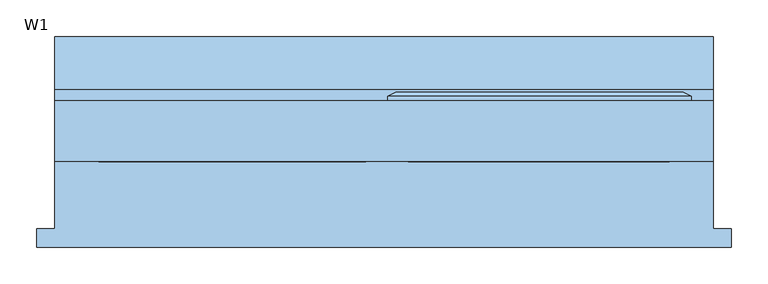
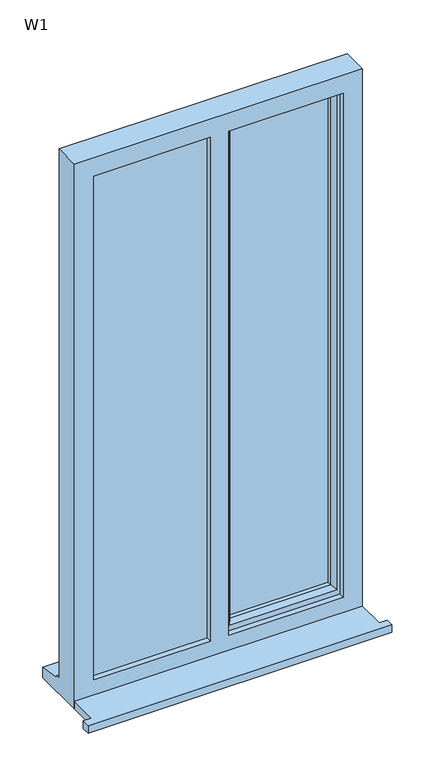
"""IFC4 building model written with IfcOpenShell, lengths in millimetres: window geometry, W1."""

from ifc_helpers import new_model, si_unit, frame, origin, place, context, project, spatial, polyline, outline, extrude, faceted_brep, source, transform, mapped, element, save


def w1_9a3d44e1(model_context):
    return source(origin(), model_context, "Body", "SolidModel", [
        extrude(outline(polyline([(-760.0, -129.0434322), (-760.0, -104.0434322), (-735.0, -104.0434322), (-735.0, -12.0434322), (165.0, -12.0434322), (165.0, -104.0434322), (190.0, -104.0434322), (190.0, -129.0434322), (-760.0, -129.0434322)])), frame((0.0, 0.0, 600.0), z_axis=(0.0, 0.0, 1.0), x_axis=(1.0, 0.0, 0.0)), (0.0, 0.0, 1.0), 25.0),
        faceted_brep([(-280.0, 70.9565678, 2370.0), (-280.0, 76.7300705, 2370.0), (-280.0, 76.7300705, 653.0), (-280.0, 70.9565678, 653.0), (-270.0, 5.9565678, 2360.0), (-270.0, 70.9565678, 2360.0), (-270.0, 70.9565678, 663.0), (-270.0, 5.9565678, 663.0), (-230.0, 20.4494677, 2320.0), (-240.1480377, 5.9565678, 2330.1480377), (-240.1480377, 5.9565678, 692.8519623), (-230.0, 20.4494677, 703.0), (-230.0, 34.9565678, 2320.0), (-230.0, 34.9565678, 703.0), (-240.0, 58.9565678, 2330.0), (-240.0, 34.9565678, 2330.0), (-240.0, 34.9565678, 693.0), (-240.0, 58.9565678, 693.0), (-230.0, 76.7300705, 2320.0), (-230.0, 58.9565678, 2320.0), (-230.0, 58.9565678, 703.0), (-230.0, 76.7300705, 703.0), (-247.4457548, 82.5035732, 2337.4457548), (-247.4457548, 82.5035732, 685.5542452), (-269.2153903, 82.5035732, 2359.2153903), (-269.2153903, 82.5035732, 663.7846097), (135.0, 76.7300705, 653.0), (135.0, 70.9565678, 653.0), (125.0, 70.9565678, 663.0), (125.0, 5.9565678, 663.0), (95.1480377, 5.9565678, 692.8519623), (85.0, 20.4494677, 703.0), (85.0, 34.9565678, 703.0), (95.0, 34.9565678, 693.0), (95.0, 58.9565678, 693.0), (85.0, 58.9565678, 703.0), (85.0, 76.7300705, 703.0), (102.4457548, 82.5035732, 685.5542452), (124.2153903, 82.5035732, 663.7846097), (135.0, 76.7300705, 2370.0), (135.0, 70.9565678, 2370.0), (125.0, 70.9565678, 2360.0), (125.0, 5.9565678, 2360.0), (95.1480377, 5.9565678, 2330.1480377), (85.0, 20.4494677, 2320.0), (85.0, 34.9565678, 2320.0), (95.0, 34.9565678, 2330.0), (95.0, 58.9565678, 2330.0), (85.0, 58.9565678, 2320.0), (85.0, 76.7300705, 2320.0), (102.4457548, 82.5035732, 2337.4457548), (124.2153903, 82.5035732, 2359.2153903)], [[[0, 1, 2, 3]], [[4, 5, 6, 7]], [[8, 9, 10, 11]], [[12, 8, 11, 13]], [[14, 15, 16, 17]], [[18, 19, 20, 21]], [[22, 18, 21, 23]], [[1, 24, 25, 2]], [[3, 2, 26, 27]], [[7, 6, 28, 29]], [[11, 10, 30, 31]], [[13, 11, 31, 32]], [[17, 16, 33, 34]], [[21, 20, 35, 36]], [[23, 21, 36, 37]], [[2, 25, 38, 26]], [[27, 26, 39, 40]], [[29, 28, 41, 42]], [[31, 30, 43, 44]], [[32, 31, 44, 45]], [[34, 33, 46, 47]], [[36, 35, 48, 49]], [[37, 36, 49, 50]], [[26, 38, 51, 39]], [[40, 39, 1, 0]], [[3, 27, 40, 0], [5, 41, 28, 6]], [[42, 41, 5, 4]], [[7, 29, 42, 4], [9, 43, 30, 10]], [[44, 43, 9, 8]], [[45, 44, 8, 12]], [[15, 46, 33, 16], [13, 32, 45, 12]], [[47, 46, 15, 14]], [[17, 34, 47, 14], [19, 48, 35, 20]], [[49, 48, 19, 18]], [[50, 49, 18, 22]], [[24, 51, 38, 25], [23, 37, 50, 22]], [[39, 51, 24, 1]]]),
        extrude(outline(polyline([(2340.0, -310.0), (2360.0, -310.0), (2360.0, -695.0), (663.0, -695.0), (663.0, -310.0), (683.0, -310.0), (683.0, -675.0), (2340.0, -675.0), (2340.0, -310.0)])), frame((0.0, 29.9565678, 0.0), z_axis=(0.0, 1.0, 0.0), x_axis=(0.0, 0.0, 1.0)), (0.0, 0.0, 1.0), 41.0),
        faceted_brep([(165.0, -12.0434322, 2400.0), (-735.0, -12.0434322, 2400.0), (-735.0, -12.0434322, 600.0), (165.0, -12.0434322, 600.0), (105.0, -12.0434322, 2340.0), (105.0, -12.0434322, 675.0), (-252.0, -12.0434322, 675.0), (-252.0, -12.0434322, 2340.0), (-310.0, -12.0434322, 2340.0), (-310.0, -12.0434322, 675.0), (-675.0, -12.0434322, 675.0), (-675.0, -12.0434322, 2340.0), (-735.0, 70.9565678, 2400.0), (-735.0, 70.9565678, 651.0), (-735.0, 85.9565678, 649.68767), (-735.0, 85.9565678, 644.7449676), (-735.0, 158.4565678, 633.8088847), (-735.0, 158.4565678, 600.0), (165.0, 70.9565678, 2400.0), (165.0, 70.9565678, 651.0), (-695.0, 70.9565678, 2360.0), (-695.0, 70.9565678, 663.0), (-310.0, 70.9565678, 663.0), (-310.0, 70.9565678, 2360.0), (-270.0, 70.9565678, 2360.0), (-270.0, 70.9565678, 663.0), (125.0, 70.9565678, 663.0), (125.0, 70.9565678, 2360.0), (-695.0, 5.9565678, 2360.0), (-695.0, 5.9565678, 663.0), (-300.0, 5.9565678, 2360.0), (-300.0, 5.9565678, 663.0), (-310.0, 5.9565678, 2340.0), (-675.0, 5.9565678, 2340.0), (-675.0, 5.9565678, 675.0), (-310.0, 5.9565678, 675.0), (-270.0, 5.9565678, 2360.0), (125.0, 5.9565678, 2360.0), (125.0, 5.9565678, 663.0), (-270.0, 5.9565678, 663.0), (105.0, 5.9565678, 2340.0), (-252.0, 5.9565678, 2340.0), (-252.0, 5.9565678, 675.0), (105.0, 5.9565678, 675.0), (-310.0, 29.9565678, 2360.0), (-300.0, 29.9565678, 2360.0), (165.0, 158.4565678, 600.0), (165.0, 158.4565678, 633.8088847), (165.0, 85.9565678, 644.7449676), (165.0, 85.9565678, 649.68767), (-300.0, 29.9565678, 663.0), (-310.0, 29.9565678, 663.0)], [[[0, 1, 2, 3], [4, 5, 6, 7], [8, 9, 10, 11]], [[2, 1, 12, 13, 14, 15, 16, 17]], [[13, 12, 18, 19], [20, 21, 22, 23], [24, 25, 26, 27]], [[21, 20, 28, 29]], [[28, 30, 31, 29], [32, 33, 34, 35]], [[36, 37, 38, 39], [40, 41, 42, 43]], [[33, 11, 10, 34]], [[1, 0, 18, 12]], [[28, 20, 23, 44, 45, 30]], [[27, 37, 36, 24]], [[11, 33, 32, 8]], [[40, 4, 7, 41]], [[19, 18, 0, 3, 46, 47, 48, 49]], [[27, 26, 38, 37]], [[4, 40, 43, 5]], [[45, 50, 31, 30]], [[50, 45, 44, 51]], [[51, 44, 23, 22]], [[25, 24, 36, 39]], [[41, 7, 6, 42]], [[8, 32, 35, 9]], [[46, 3, 2, 17]], [[47, 46, 17, 16]], [[48, 47, 16, 15]], [[49, 48, 15, 14]], [[19, 49, 14, 13]], [[22, 21, 29, 31, 50, 51]], [[26, 25, 39, 38]], [[6, 5, 43, 42]], [[35, 34, 10, 9]]]),
        extrude(outline(polyline([(-695.0, 29.9565678), (-300.0, 29.9565678), (-300.0, 5.9565678), (-695.0, 5.9565678), (-695.0, 29.9565678)])), frame((0.0, 0.0, 663.0), z_axis=(0.0, 0.0, 1.0), x_axis=(1.0, 0.0, 0.0)), (0.0, 0.0, 1.0), 1697.0),
        extrude(outline(polyline([(95.0, 34.9565678), (-240.0, 34.9565678), (-240.0, 58.9565678), (95.0, 58.9565678), (95.0, 34.9565678)])), frame((0.0, 0.0, 693.0), z_axis=(0.0, 0.0, 1.0), x_axis=(1.0, 0.0, 0.0)), (0.0, 0.0, 1.0), 1637.0),
    ])


if __name__ == "__main__":
    model = new_model("IFC4")
    model_context = context("Model", 3, world=origin())
    ifc_project = project(units=[si_unit("LENGTHUNIT", "METRE", prefix="MILLI")], contexts=[model_context])
    site = spatial("IfcSite", under=ifc_project)
    building = spatial("IfcBuilding", under=site)
    placement = place(None, origin())
    w1_shape = w1_9a3d44e1(model_context)
    element("IfcWindow", 1, ObjectType="W1", at=placement, inside=building, context=model_context, shape_type="MappedRepresentation", body=[
        mapped(w1_shape, transform((0.0, 0.0, 0.0), x_axis=(1.0, 0.0, 0.0), y_axis=(0.0, 1.0, 0.0), z_axis=(0.0, 0.0, 1.0))),
    ])
    save(model, "model.ifc")

# Revit data of these elements
# Type "W1"
#   Type Mark = "40"
#   Operation = "DoublePanelVertical"
#   Manufacturer = "Revit"
#   Wrap Layers (Ext) from Ext = 102.5 mm
#   Wrap Layers (Int) from Ext = 177.5 mm
#   Window Board Projection = 25 mm
#   Window Board Extension = 25 mm
#   Rough Width = 900 mm
#   Rough Height = 1800 mm
#   Height = 1800 mm
#   Width = 900 mm
#   Glazing Thickness = 24 mm
#   FrameOffset - External = 50 mm
#   Frame Depth = 65 mm
#   Default Head Height = 2400 mm
#   Cill Depth = 87.5 mm
#   Cavity Closer Width = 50 mm
#   Cavity Closer Offset from Ext = 102.5 mm
#   Cavity Closer Depth = 85 mm
#   Vis - Cavity Closers = yes
#   Material Trim = Window Frame
#   Material Glass = Glass
#   Material Frame = Window Frame
#   Wall Closure = (empty or 0)
# Element 1 (IfcWindow, "W1")
#   Materials on its faces: "Window Frame", "Glass"
# Materials
#   "Window Frame": colour RGB 249 249 249, transparency 0
#   "Glass": class "Glass", colour RGB 245 245 243, transparency 1, Description = "Soda Lime Glass", Cost = 0
